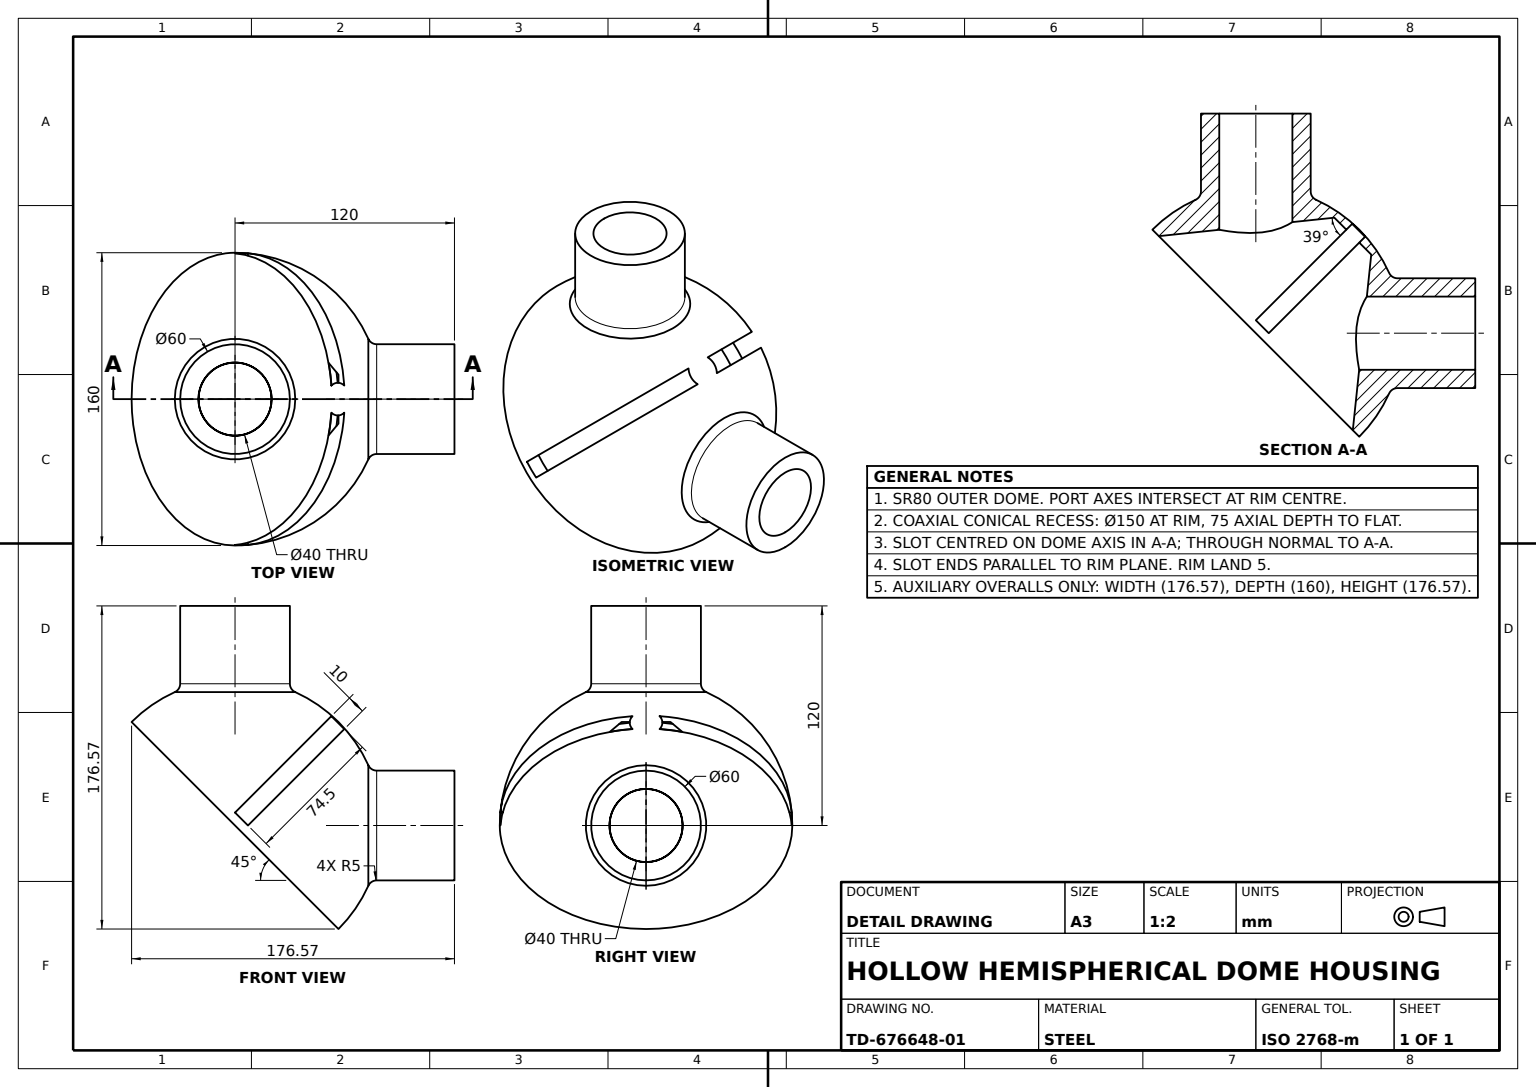
SolidWorks part; units mm, degrees
material "Plain Carbon Steel"
ref_plane "Front Plane" through (0, 0, 0) normal (0, 0, 1) x (1, 0, 0)
ref_plane "Top Plane" through (0, 0, 0) normal (0, 1, 0) x (1, 0, 0)
ref_plane "Right Plane" through (0, 0, 0) normal (1, 0, 0) x (0, 0, -1)
sketch "Dome Profile Sketch" plane through (0, 0, 0) normal (0, 0, 1) x (1, 0, 0)
  line L0 (0, 0) -> (0, 80)
  line L1 (0, 0) -> (80, 0)
  arc A0 (0, 80) -> (80, 0) centre (0, 0) cw
  dimension "D1" = 80
  dimension "D3" = 80
  dimension "D2" = 80
revolve "Dome R80" add sketch "Dome Profile Sketch" angle 360 about L0
ref_plane "Slot Sketch Plane" through (0, 0, 0) normal (1, 0, 0) x (0, 0, -1)
sketch "Dome Slot Sketch" plane through (0, 0, 0) normal (1, 0, 0) x (0, 0, -1)
  line L2 (5, 75) -> (5, 5)
  line L3 (5, 78) -> (5, 79.5)
  line L5 (-5, 5) -> (-5, 75)
  line L7 (-5, 5) -> (5, 5)
  line L9 (-5, 75) -> (-5, 78)
  line L11 (5, 78) -> (5, 75)
  line L12 (-5, 78) -> (-5, 79)
  line L13 (5, 79.5) -> (-5, 79.5)
  line L14 (-5, 79.5) -> (-5, 79)
  dimension "D1" = 5
  dimension "D2" = 5
  dimension "D3" = 10
  dimension "D4" = 5
  dimension "D5" = 70
  dimension "D6" = 73
  dimension "D7" = 74
  dimension "D8" = 74.5
extrude "Dome Slot Cut" cut sketch "Dome Slot Sketch" against normal mid plane 210
sketch "Angled Cut Sketch" plane through (0, 0, 0) normal (0, -1, 0) x (1, 0, 0)
  circle A0 centre (0, 0) radius 75
  dimension "D1" = 150
extrude "Angled Cut" cut sketch "Angled Cut Sketch" against normal blind 75 draft 39
sketch "Tube Boss Profile Sketch" plane through (0, 0, 0) normal (1, 0, 0) x (0, 0, -1)
  line L0 (47.6943, 47.6943) -> (84.8528, 84.8528)
  line L1 (84.8528, 84.8528) -> (106.066, 63.6396)
  line L2 (106.066, 63.6396) -> (68.9075, 26.4811)
  line L3 (68.9075, 26.4811) -> (50.8002, 44.5884)
  line L4 (50.8002, 44.5884) -> (47.6943, 47.6943)
  dimension "D1" = 120
  dimension "D2" = 30
  dimension "D3" = 52.5501
  dimension "D4" = 4.3924
  dimension "D5" = 84.8528
revolve "Tube Boss" add sketch "Tube Boss Profile Sketch" angle 360 about L0
ref_plane "Tube Bore Plane" through (0, 84.8528, -84.8528) normal (0, 0.7071, -0.7071) x (1, 0, 0)
sketch "Tube Bore Sketch" plane through (0, 84.8528, -84.8528) normal (0, 0.7071, -0.7071) x (1, 0, 0)
  circle A0 centre (0, 0) radius 20
  dimension "D1" = 40
extrude "Tube Bore Cut" cut sketch "Tube Bore Sketch" against normal blind 75
mirror "Tube Bore Mirror" about plane through (0, 0, 0) normal (0, 0, 1) of "Tube Bore Cut", "Tube Boss"
fillet "Tube Fillet R5" radius 5 2 edges at (0, 31.2272, -73.6536) (0, 73.6536, 31.2272)
